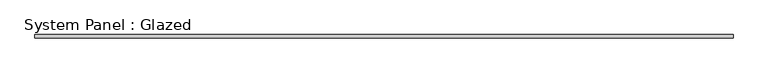
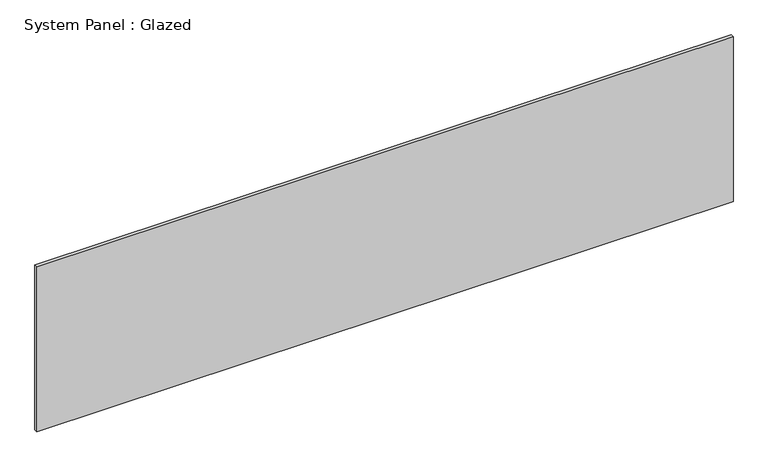
"""IFC4 building model written with IfcOpenShell, lengths in millimetres: plate geometry, System Panel : Glazed."""

from ifc_helpers import new_model, si_unit, origin, origin_with_axes, place, context, project, spatial, polyline, outline, extrude, source, transform, mapped, element, save


def system_panel_glazed_b08977a1(model_context):
    return source(origin(), model_context, "Body", "SweptSolid", [
        extrude(outline(polyline([(2705.6657817, 19.05), (-2705.6657817, 19.05), (-2705.6657817, 44.45), (2705.6657817, 44.45), (2705.6657817, 19.05)])), origin_with_axes(), (0.0, 0.0, 1.0), 1355.563107),
    ])


if __name__ == "__main__":
    model = new_model("IFC4")
    model_context = context("Model", 3, world=origin())
    ifc_project = project(units=[si_unit("LENGTHUNIT", "METRE", prefix="MILLI")], contexts=[model_context])
    site = spatial("IfcSite", under=ifc_project)
    building = spatial("IfcBuilding", under=site)
    placement = place(None, origin())
    system_panel_glazed_shape = system_panel_glazed_b08977a1(model_context)
    element("IfcPlate", 1, ObjectType="System Panel : Glazed", at=placement, inside=building, context=model_context, shape_type="MappedRepresentation", body=[
        mapped(system_panel_glazed_shape, transform((0.0, 0.0, 0.0), x_axis=(1.0, 0.0, 0.0), y_axis=(0.0, 1.0, 0.0), z_axis=(0.0, 0.0, 1.0))),
    ])
    save(model, "model.ifc")

# Revit data of these elements
# Type "System Panel : Glazed"
#   Construction Type Id = "GSP4R"
#   Analytic Construction = "1/8 in Pilkington single glazing"
#   Visual Light Transmittance = 0.9
#   Solar Heat Gain Coefficient = 0.86
#   Heat Transfer Coefficient (U) = 1.18115 BTU/(h·ft²·°F)
#   Define Thermal Properties by = 1
# Element 1 (IfcPlate, "System Panel : Glazed")
#   Materials on its faces: "Glass"
# Materials
#   "Glass": class "Glass", colour RGB 0 128 192, transparency 0.75, Description = "Soda Lime Glass", Cost = 0
